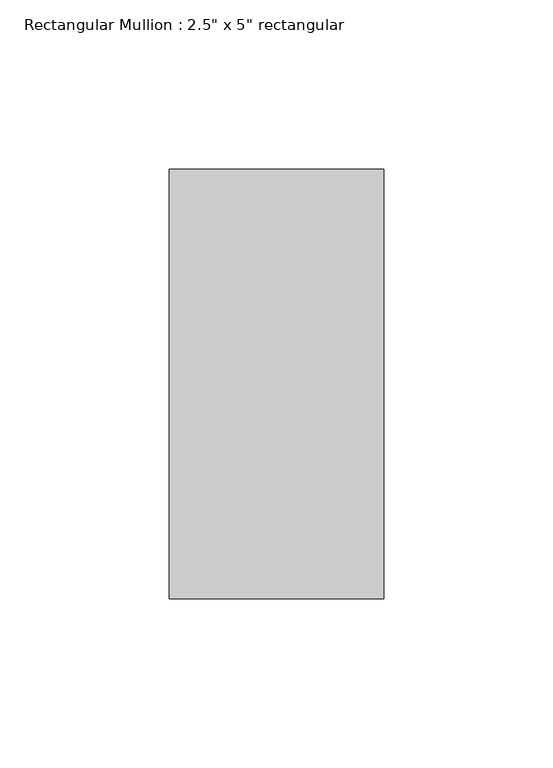
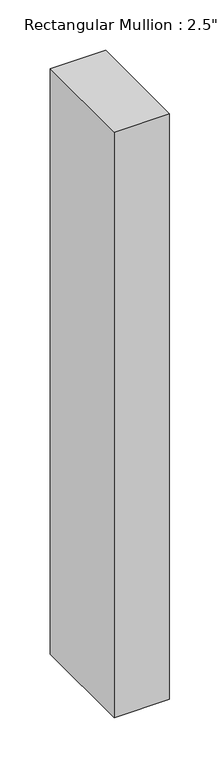
"""IFC4 building model written with IfcOpenShell, lengths in millimetres: member geometry."""

from ifc_helpers import new_model, si_unit, frame, origin, place, context, project, spatial, polyline, outline, extrude, source, transform, mapped, element, save


def member_ae70dd35(model_context):
    return source(origin(), model_context, "Body", "SweptSolid", [
        extrude(outline(polyline([(0.0, 63.5), (0.0, -63.5), (-63.5, -63.5), (-63.5, 63.5), (0.0, 63.5)])), frame((0.0, 0.0, -711.2), z_axis=(0.0, 0.0, 1.0), x_axis=(1.0, 0.0, 0.0)), (0.0, 0.0, 1.0), 711.2),
    ])


if __name__ == "__main__":
    model = new_model("IFC4")
    model_context = context("Model", 3, world=origin())
    ifc_project = project(units=[si_unit("LENGTHUNIT", "METRE", prefix="MILLI")], contexts=[model_context])
    site = spatial("IfcSite", under=ifc_project)
    building = spatial("IfcBuilding", under=site)
    placement = place(None, origin())
    member_shape = member_ae70dd35(model_context)
    element("IfcMember", 1, ObjectType="Rectangular Mullion : 2.5\" x 5\" rectangular", at=placement, inside=building, context=model_context, shape_type="MappedRepresentation", body=[
        mapped(member_shape, transform((0.0, 0.0, 0.0), x_axis=(1.0, 0.0, 0.0), y_axis=(0.0, 1.0, 0.0), z_axis=(0.0, 0.0, 1.0))),
    ])
    save(model, "model.ifc")

# Revit data of these elements
# Type "Rectangular Mullion : 2.5\" x 5\" rectangular"
#   built-in parameter 1007304 = 0.416667 (stored number, unit not read)
#   built-in parameter 1007301 = 0.104167 (stored number, unit not read)
#   built-in parameter 1007300 = 0.104167 (stored number, unit not read)
# Element 1 (IfcMember, "Rectangular Mullion : 2.5\" x 5\" rectangular")
#   Materials on its faces: "Aluminum"
# Materials
#   "Aluminum": class "Metal", colour RGB 247 247 247, transparency 0, Description = "Aluminum 6061", Cost = 0
